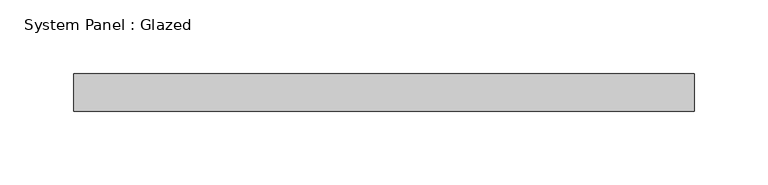
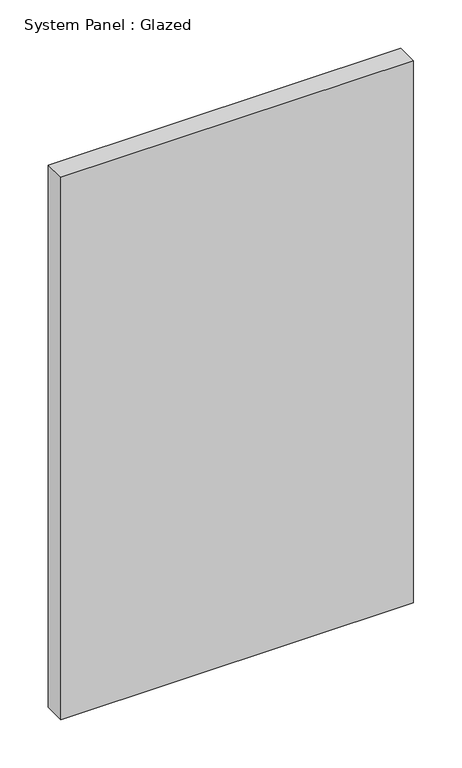
"""IFC4 building model written with IfcOpenShell, lengths in millimetres: plate geometry, System Panel : Glazed."""

from ifc_helpers import new_model, si_unit, origin, origin_with_axes, place, context, project, spatial, polyline, outline, extrude, source, transform, mapped, element, save


def system_panel_glazed_5fd0c891(model_context):
    return source(origin(), model_context, "Body", "SweptSolid", [
        extrude(outline(polyline([(210.6083333, 19.05), (-210.6083333, 19.05), (-210.6083333, 44.45), (210.6083333, 44.45), (210.6083333, 19.05)])), origin_with_axes(), (0.0, 0.0, 1.0), 684.9785678),
    ])


if __name__ == "__main__":
    model = new_model("IFC4")
    model_context = context("Model", 3, world=origin())
    ifc_project = project(units=[si_unit("LENGTHUNIT", "METRE", prefix="MILLI")], contexts=[model_context])
    site = spatial("IfcSite", under=ifc_project)
    building = spatial("IfcBuilding", under=site)
    placement = place(None, origin())
    system_panel_glazed_shape = system_panel_glazed_5fd0c891(model_context)
    element("IfcPlate", 1, ObjectType="System Panel : Glazed", at=placement, inside=building, context=model_context, shape_type="MappedRepresentation", body=[
        mapped(system_panel_glazed_shape, transform((0.0, 0.0, 0.0), x_axis=(1.0, 0.0, 0.0), y_axis=(0.0, 1.0, 0.0), z_axis=(0.0, 0.0, 1.0))),
    ])
    save(model, "model.ifc")

# Revit data of these elements
# Type "System Panel : Glazed"
#   Construction Type Id = "GSP4R"
#   Analytic Construction = "1/8 in Pilkington single glazing"
#   Visual Light Transmittance = 0.9
#   Solar Heat Gain Coefficient = 0.86
#   Heat Transfer Coefficient (U) = 1.18115 BTU/(h·ft²·°F)
#   Define Thermal Properties by = 1
# Element 1 (IfcPlate, "System Panel : Glazed")
#   Materials on its faces: "Glass"
# Materials
#   "Glass": class "Glass", colour RGB 0 128 192, transparency 0.75, Description = "Soda Lime Glass", Cost = 0
